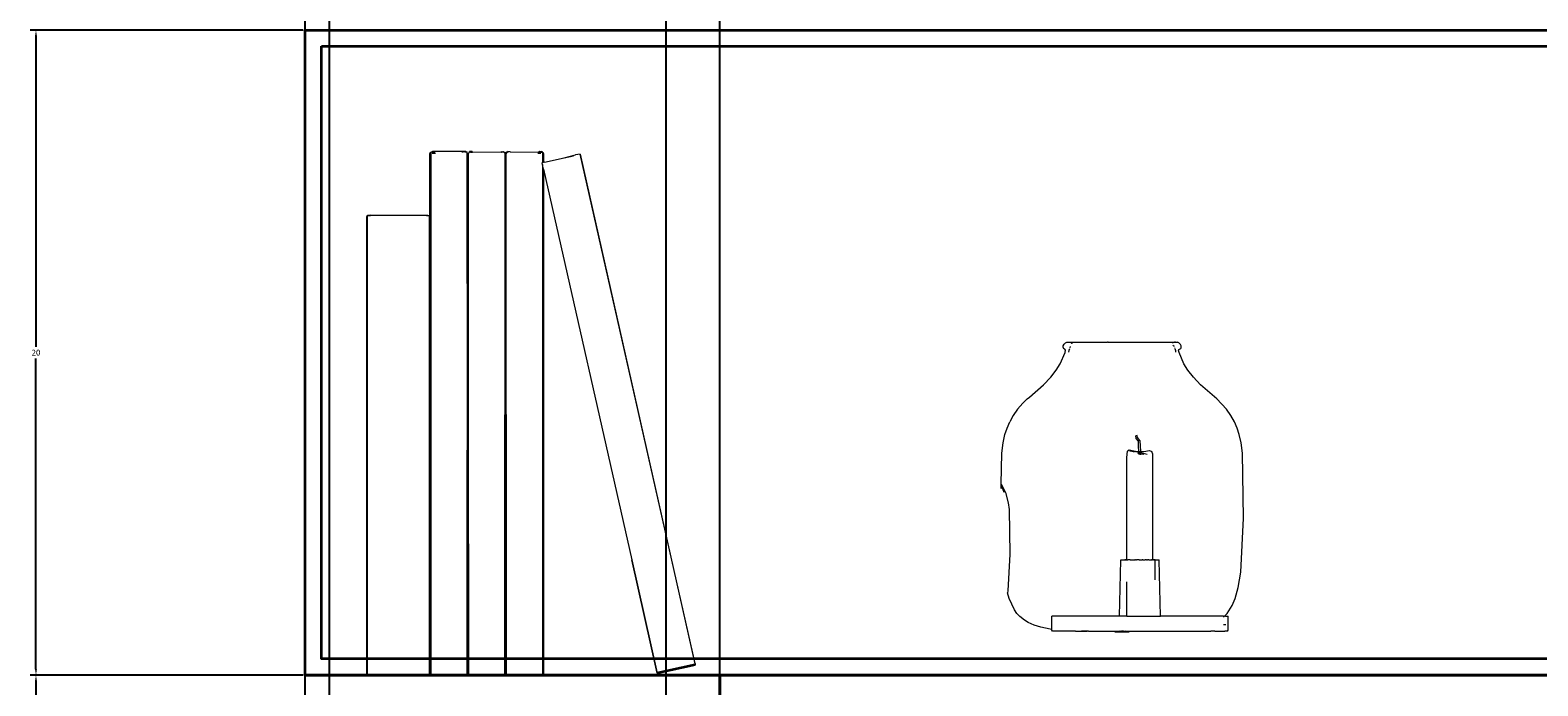
# Model space of a CAD drawing. Units: millimetres. Extents: x 446512 to 447461, y 70395 to 70610.
# Tile 18 of 39: x 446678 to 446725, y 70513 to 70533. Entities that reach past the tile are written whole.
import ezdxf

# ---------------------------------------------------------------- set-up
doc = ezdxf.new("R2010")
doc.units = ezdxf.units.MM
for name, color, linetype, lineweight in [('A-ANNO-DIMS', 2, 'Continuous', 18), ('A-CONS', 9, 'Continuous', 13), ('A-FURN', 7, 'Continuous', 35), ('A-FURN-DECO', 8, 'Continuous', 13)]:
    doc.layers.add(name, color=color, linetype=linetype, lineweight=lineweight)
doc.styles.get("Standard").update_dxf_attribs({"font": 'arial.ttf'})
doc.dimstyles.get("Standard").update_dxf_attribs({"dimtxt": 0.18, "dimasz": 0.18, "dimexe": 0.18, "dimexo": 0.0625, "dimgap": 0.09, "dimtad": 0, "dimtih": 1, "dimtoh": 1, "dimdec": 4, "dimzin": 0, "dimdsep": 46, "dimtxsty": 'Standard', "dimcen": 0.09, "dimadec": 0, "dimazin": 0, "dimtfac": 1, "dimtdec": 4, "dimtofl": 0, "dimtmove": 0, "dimatfit": 3, "dimfxl": 1, "dimtolj": 1, "dimtzin": 0, "dimarcsym": 0})

# ---------------------------------------------------------------- blocks, each defined once
blk = doc.blocks.new('DECO-VASE-A')
for p, q in [((1.923, 8.866), (1.951, 8.922)), ((1.951, 8.922), (1.992, 8.962)), ((1.992, 8.962), (2.04, 8.983)), ((2.04, 8.983), (2.147, 8.974)), ((2.04, 8.983), (3.3, 8.983)), ((2.147, 8.974), (2.186, 8.942)), ((2.186, 8.942), (2.19, 8.923)), ((3.314, 8.982), (3.3, 8.983)), ((3.314, 8.982), (5.399, 8.983)), ((5.308, 8.977), (5.375, 8.979)), ((5.332, 8.964), (5.314, 8.943)), ((5.325, 8.885), (5.351, 8.865)), ((5.375, 8.979), (5.332, 8.964)), ((5.399, 8.983), (5.375, 8.979)), ((5.403, 8.983), (5.399, 8.983)), ((5.403, 8.983), (5.462, 8.982)), ((5.511, 8.96), (5.462, 8.982)), ((5.56, 8.904), (5.511, 8.96)), ((5.576, 8.866), (5.56, 8.904)), ((1.832, 8.302), (1.985, 8.655)), ((1.917, 8.815), (1.923, 8.866)), ((1.917, 8.815), (1.931, 8.786)), ((1.974, 8.762), (1.931, 8.786)), ((1.996, 8.731), (1.974, 8.762)), ((1.985, 8.655), (1.996, 8.731)), ((2.1, 8.723), (2.091, 8.673)), ((2.115, 8.769), (2.1, 8.723)), ((2.141, 8.848), (2.125, 8.798)), ((5.351, 8.865), (5.358, 8.847)), ((5.373, 8.802), (5.377, 8.793)), ((5.382, 8.778), (5.4, 8.725)), ((5.4, 8.725), (5.409, 8.672)), ((5.503, 8.731), (5.511, 8.747)), ((5.515, 8.655), (5.503, 8.731)), ((5.511, 8.747), (5.566, 8.783)), ((5.668, 8.302), (5.515, 8.655)), ((5.566, 8.783), (5.581, 8.808)), ((5.581, 8.808), (5.576, 8.866)), ((1.541, 7.898), (1.71, 8.114)), ((1.71, 8.114), (1.832, 8.302)), ((5.789, 8.114), (5.668, 8.302)), ((5.959, 7.898), (5.789, 8.114)), ((0.874, 7.277), (1.315, 7.659)), ((1.315, 7.659), (1.541, 7.898)), ((6.185, 7.659), (5.959, 7.898)), ((6.689, 7.222), (6.185, 7.659)), ((0.508, 6.898), (0.67, 7.084)), ((0.67, 7.084), (0.81, 7.222)), ((0.81, 7.222), (0.874, 7.277)), ((6.991, 6.898), (6.689, 7.222)), ((0.375, 6.707), (0.267, 6.512)), ((0.508, 6.898), (0.375, 6.707)), ((7.124, 6.707), (6.991, 6.898)), ((7.232, 6.512), (7.124, 6.707)), ((0.06, 5.856), (0.117, 6.113)), ((0.117, 6.113), (0.182, 6.314)), ((0.182, 6.314), (0.267, 6.512)), ((4.217, 6.081), (4.173, 6.078)), ((4.184, 5.991), (4.173, 6.078)), ((4.227, 6.021), (4.217, 6.081)), ((7.317, 6.314), (7.232, 6.512)), ((7.382, 6.113), (7.317, 6.314)), ((7.44, 5.856), (7.382, 6.113)), ((0.02, 5.541), (0.06, 5.856)), ((3.97, 5.625), (3.916, 5.6)), ((4.168, 5.588), (3.97, 5.625)), ((4.129, 5.567), (3.989, 5.611)), ((3.989, 5.611), (4.168, 5.588)), ((4.258, 5.909), (4.184, 5.991)), ((4.297, 5.928), (4.227, 6.021)), ((4.261, 5.759), (4.258, 5.909)), ((4.266, 5.588), (4.261, 5.759)), ((4.297, 5.928), (4.32, 5.588)), ((4.422, 5.588), (4.602, 5.615)), ((4.602, 5.615), (4.675, 5.587)), ((7.479, 5.541), (7.44, 5.856)), ((0.002, 4.579), (0.02, 5.541)), ((3.893, 5.401), (3.916, 5.6)), ((3.893, 2.225), (3.893, 5.401)), ((4.168, 5.588), (4.266, 5.588)), ((4.267, 5.562), (4.168, 5.588)), ((4.268, 5.524), (4.24, 5.533)), ((4.267, 5.562), (4.266, 5.588)), ((4.266, 5.588), (4.32, 5.588)), ((4.322, 5.548), (4.267, 5.562)), ((4.267, 5.554), (4.267, 5.559)), ((4.268, 5.524), (4.267, 5.541)), ((4.295, 5.515), (4.268, 5.524)), ((4.268, 5.504), (4.268, 5.524)), ((4.303, 5.503), (4.268, 5.504)), ((4.295, 5.515), (4.325, 5.513)), ((4.303, 5.503), (4.325, 5.502)), ((4.32, 5.588), (4.322, 5.548)), ((4.32, 5.588), (4.422, 5.588)), ((4.525, 5.496), (4.322, 5.548)), ((4.323, 5.541), (4.324, 5.523)), ((4.325, 5.513), (4.325, 5.502)), ((4.325, 5.513), (4.428, 5.504)), ((4.691, 5.523), (4.675, 5.587)), ((4.691, 5.523), (4.695, 2.225)), ((7.516, 3.52), (7.479, 5.541)), ((0, 4.513), (0.002, 4.579)), ((0.002, 4.51), (0, 4.513)), ((0, 4.439), (0.002, 4.51)), ((0.002, 4.579), (0.134, 4.312)), ((0.052, 4.428), (0.002, 4.51)), ((0.095, 4.312), (0.052, 4.428)), ((0.134, 4.312), (0.217, 3.999)), ((0.217, 3.999), (0.244, 3.785)), ((0.244, 3.785), (0.269, 2.409)), ((7.431, 1.848), (7.516, 3.52)), ((0.269, 2.409), (0.211, 1.27)), ((3.665, 0.487), (3.705, 2.219)), ((3.705, 2.219), (3.712, 2.225)), ((3.712, 2.225), (3.763, 2.225)), ((3.763, 2.225), (3.766, 2.225)), ((3.766, 2.225), (3.789, 2.225)), ((3.789, 2.225), (3.795, 2.225)), ((3.795, 2.225), (3.797, 2.225)), ((3.797, 2.225), (3.813, 2.225)), ((3.813, 2.225), (3.821, 2.225)), ((3.821, 2.225), (3.825, 2.225)), ((3.825, 2.225), (3.828, 2.225)), ((3.828, 2.225), (3.832, 2.225)), ((3.832, 2.225), (3.838, 2.225)), ((3.842, 2.225), (3.838, 2.225)), ((3.838, 2.225), (3.838, 2.219)), ((3.842, 2.225), (3.844, 2.225)), ((3.844, 2.225), (3.852, 2.225)), ((3.864, 2.225), (3.852, 2.225)), ((3.867, 2.225), (3.864, 2.225)), ((3.867, 2.225), (3.878, 2.225)), ((3.878, 2.225), (3.881, 2.225)), ((3.881, 2.225), (3.883, 2.225)), ((3.883, 2.225), (3.893, 2.225)), ((3.893, 2.219), (3.893, 2.225)), ((3.908, 2.225), (3.893, 2.225)), ((3.908, 2.225), (3.927, 2.225)), ((3.992, 2.225), (3.927, 2.225)), ((4.002, 2.225), (3.992, 2.225)), ((4.002, 2.225), (4.053, 2.225)), ((4.053, 2.225), (4.065, 2.225)), ((4.065, 2.225), (4.148, 2.225)), ((4.163, 2.225), (4.148, 2.225)), ((4.163, 2.225), (4.192, 2.225)), ((4.278, 2.225), (4.192, 2.225)), ((4.278, 2.225), (4.283, 2.225)), ((4.283, 2.225), (4.374, 2.225)), ((4.394, 2.225), (4.374, 2.225)), ((4.394, 2.225), (4.451, 2.225)), ((4.451, 2.225), (4.462, 2.225)), ((4.496, 2.225), (4.462, 2.225)), ((4.5, 2.225), (4.496, 2.225)), ((4.505, 2.225), (4.5, 2.225)), ((4.505, 2.225), (4.508, 2.225)), ((4.508, 2.225), (4.511, 2.225)), ((4.511, 2.225), (4.541, 2.225)), ((4.553, 2.225), (4.541, 2.225)), ((4.578, 2.225), (4.553, 2.225)), ((4.578, 2.225), (4.583, 2.225)), ((4.583, 2.225), (4.65, 2.225)), ((4.659, 2.225), (4.65, 2.225)), ((4.659, 2.225), (4.683, 2.225)), ((4.69, 2.225), (4.683, 2.225)), ((4.695, 2.225), (4.69, 2.225)), ((4.695, 2.225), (4.695, 2.219)), ((4.697, 2.225), (4.695, 2.225)), ((4.702, 2.225), (4.697, 2.225)), ((4.704, 2.225), (4.702, 2.225)), ((4.704, 2.225), (4.718, 2.225)), ((4.722, 2.225), (4.718, 2.225)), ((4.74, 2.225), (4.722, 2.225)), ((4.744, 2.225), (4.74, 2.225)), ((4.744, 2.225), (4.756, 2.225)), ((4.769, 2.225), (4.756, 2.225)), ((4.769, 2.225), (4.76, 1.611)), ((4.773, 2.225), (4.769, 2.225)), ((4.777, 2.225), (4.773, 2.225)), ((4.777, 2.225), (4.802, 2.225)), ((4.802, 2.225), (4.807, 2.225)), ((4.807, 2.225), (4.813, 2.225)), ((4.813, 2.225), (4.834, 2.225)), ((4.834, 2.225), (4.837, 2.225)), ((4.837, 2.225), (4.84, 2.225)), ((4.84, 2.225), (4.849, 2.225)), ((4.849, 2.225), (4.895, 2.225)), ((4.902, 2.219), (4.895, 2.225)), ((4.942, 0.487), (4.902, 2.219)), ((3.893, 0.487), (3.893, 1.548)), ((7.347, 1.371), (7.431, 1.848)), ((0.211, 1.27), (0.2, 1.204)), ((0.248, 1.032), (0.2, 1.204)), ((0.41, 0.681), (0.248, 1.032)), ((7.16, 0.81), (7.251, 1.032)), ((7.251, 1.032), (7.347, 1.371)), ((0.488, 0.567), (0.41, 0.681)), ((0.576, 0.472), (0.488, 0.567)), ((0.727, 0.355), (0.576, 0.472)), ((1.567, 0.24), (1.568, 0.487)), ((3.665, 0.487), (1.568, 0.487)), ((3.893, 0.487), (3.665, 0.487)), ((3.893, 0.487), (4.942, 0.487)), ((6.889, 0.487), (4.942, 0.487)), ((6.889, 0.452), (6.926, 0.487)), ((6.889, 0.487), (6.926, 0.487)), ((6.926, 0.487), (7.011, 0.567)), ((6.938, 0.487), (6.926, 0.487)), ((6.953, 0.487), (6.938, 0.487)), ((6.953, 0.487), (7.039, 0.487)), ((7.011, 0.567), (7.16, 0.81)), ((7.039, 0.045), (7.039, 0.487)), ((0.839, 0.288), (0.727, 0.355)), ((1.025, 0.205), (0.839, 0.288)), ((1.227, 0.14), (1.025, 0.205)), ((1.518, 0.077), (1.227, 0.14)), ((1.567, 0.071), (1.518, 0.077)), ((1.567, 0.071), (1.567, 0.24)), ((1.567, 0.045), (1.567, 0.071)), ((1.588, 0.02), (1.567, 0.045)), ((2.274, 0.02), (1.588, 0.02)), ((2.295, 0.021), (2.274, 0.02)), ((2.306, 0.02), (2.295, 0.021)), ((2.306, 0.02), (2.665, 0.02)), ((2.665, 0.02), (2.495, 0.021)), ((2.684, 0.022), (2.665, 0.02)), ((2.704, 0.02), (2.684, 0.022)), ((2.704, 0.02), (3.676, 0.02)), ((3.521, 0), (3.685, 0.017)), ((3.521, 0), (3.97, 0)), ((3.685, 0.017), (3.676, 0.02)), ((3.685, 0.017), (3.729, 0.02)), ((3.775, 0.017), (3.729, 0.02)), ((3.793, 0.02), (3.775, 0.017)), ((3.793, 0.02), (3.84, 0.017)), ((3.84, 0.017), (3.859, 0.02)), ((3.97, 0), (3.84, 0.017)), ((3.859, 0.02), (6.333, 0.02)), ((6.333, 0.02), (6.501, 0.021)), ((6.622, 0.02), (6.501, 0.021)), ((6.622, 0.02), (6.643, 0.02)), ((6.643, 0.02), (6.645, 0.02)), ((6.643, 0.02), (6.647, 0.02)), ((6.647, 0.02), (6.749, 0.02)), ((6.749, 0.02), (6.768, 0.02)), ((6.768, 0.02), (6.77, 0.02)), ((6.77, 0.02), (6.854, 0.02)), ((6.854, 0.02), (6.911, 0.02)), ((6.911, 0.02), (6.933, 0.02)), ((6.945, 0.02), (6.933, 0.02)), ((7.019, 0.02), (6.945, 0.02)), ((7.019, 0.02), (7.039, 0.045))]:
    blk.add_line(p, q)
blk = doc.blocks.new('*D22')
at = {"layer": 'A-ANNO-DIMS', "color": 0, "lineweight": -2, "transparency": 16777216}
for p, q in [((446686.51, 70513.382), (446678.043, 70513.382)), ((446678.223, 70513.202), (446678.223, 70503.563)), ((446678.223, 70493.562), (446678.223, 70503.2)), ((446686.51, 70493.382), (446678.043, 70493.382))]:
    blk.add_line(p, q, dxfattribs=at)
at = {"layer": 'A-ANNO-DIMS', "color": 0, "transparency": 16777216}
for points in [[(446678.193, 70513.202), (446678.253, 70513.202), (446678.223, 70513.382)], [(446678.193, 70493.562), (446678.253, 70493.562), (446678.223, 70493.382)]]:
    blk.add_solid(points, dxfattribs=at)
at = {"layer": 'Defpoints', "color": 0, "transparency": 16777216}
for p in [(446678.223, 70513.382), (446686.573, 70513.382), (446686.573, 70493.382)]:
    blk.add_point(p, dxfattribs=at)
at = {"layer": 'A-ANNO-DIMS', "color": 0, "transparency": 16777216, "insert": (446678.223, 70503.382), "char_height": 0.18, "attachment_point": 5}
blk.add_mtext('\\A1;20', dxfattribs=at)
blk = doc.blocks.new('*D23')
at = {"layer": 'A-ANNO-DIMS', "color": 0, "lineweight": -2, "transparency": 16777216}
for p, q in [((446686.51, 70533.382), (446678.043, 70533.382)), ((446678.223, 70533.202), (446678.223, 70523.563)), ((446678.223, 70513.562), (446678.223, 70523.2)), ((446686.51, 70513.382), (446678.043, 70513.382))]:
    blk.add_line(p, q, dxfattribs=at)
at = {"layer": 'A-ANNO-DIMS', "color": 0, "transparency": 16777216}
for points in [[(446678.193, 70533.202), (446678.253, 70533.202), (446678.223, 70533.382)], [(446678.193, 70513.562), (446678.253, 70513.562), (446678.223, 70513.382)]]:
    blk.add_solid(points, dxfattribs=at)
at = {"layer": 'Defpoints', "color": 0, "transparency": 16777216}
for p in [(446678.223, 70533.382), (446686.573, 70533.382), (446686.573, 70513.382)]:
    blk.add_point(p, dxfattribs=at)
at = {"layer": 'A-ANNO-DIMS', "color": 0, "transparency": 16777216, "insert": (446678.223, 70523.382), "char_height": 0.18, "attachment_point": 5}
blk.add_mtext('\\A1;20', dxfattribs=at)
blk = doc.blocks.new('*D37')
at = {"layer": 'A-ANNO-DIMS', "color": 0, "lineweight": -2, "transparency": 16777216}
for p, q in [((446686.572846, 70433.44405), (446686.572846, 70578.17492)), ((446687.323552, 70428.838404), (446687.323552, 70578.17492)), ((446686.392846, 70577.99492), (446686.212846, 70577.99492)), ((446687.503552, 70577.99492), (446687.683552, 70577.99492))]:
    blk.add_line(p, q, dxfattribs=at)
at = {"layer": 'A-ANNO-DIMS', "color": 0, "transparency": 16777216}
for points in [[(446686.392846, 70578.02492), (446686.392846, 70577.96492), (446686.572846, 70577.99492)], [(446687.503552, 70578.02492), (446687.503552, 70577.96492), (446687.323552, 70577.99492)]]:
    blk.add_solid(points, dxfattribs=at)
at = {"layer": 'Defpoints', "color": 0, "transparency": 16777216}
for p in [(446687.323552, 70577.99492), (446686.572846, 70433.38155), (446687.323552, 70428.775904)]:
    blk.add_point(p, dxfattribs=at)
at = {"layer": 'A-ANNO-DIMS', "color": 0, "transparency": 16777216, "insert": (446686.948199, 70577.99492), "char_height": 0.18, "attachment_point": 5}
blk.add_mtext('\\A1;0.75', dxfattribs=at)
blk = doc.blocks.new('*D38')
at = {"layer": 'A-ANNO-DIMS', "color": 0, "lineweight": -2, "transparency": 16777216}
for p, q in [((446687.323552, 70428.838404), (446687.323552, 70578.17492)), ((446697.765686, 70428.838404), (446697.765686, 70578.17492)), ((446687.503552, 70577.99492), (446692.090383, 70577.99492)), ((446697.585686, 70577.99492), (446692.998855, 70577.99492))]:
    blk.add_line(p, q, dxfattribs=at)
at = {"layer": 'A-ANNO-DIMS', "color": 0, "transparency": 16777216}
for points in [[(446687.503552, 70578.02492), (446687.503552, 70577.96492), (446687.323552, 70577.99492)], [(446697.585686, 70578.02492), (446697.585686, 70577.96492), (446697.765686, 70577.99492)]]:
    blk.add_solid(points, dxfattribs=at)
at = {"layer": 'Defpoints', "color": 0, "transparency": 16777216}
for p in [(446697.765686, 70577.99492), (446687.323552, 70428.775904), (446697.765686, 70428.775904)]:
    blk.add_point(p, dxfattribs=at)
at = {"layer": 'A-ANNO-DIMS', "color": 0, "transparency": 16777216, "insert": (446692.544619, 70577.99492), "char_height": 0.18, "attachment_point": 5}
blk.add_mtext('\\A1;10.442', dxfattribs=at)
blk = doc.blocks.new('*D39')
at = {"layer": 'A-ANNO-DIMS', "color": 0, "lineweight": -2, "transparency": 16777216}
for p, q in [((446697.766, 70428.838), (446697.766, 70578.175)), ((446699.429, 70433.444), (446699.429, 70578.175)), ((446697.946, 70577.995), (446698.212, 70577.995)), ((446699.249, 70577.995), (446698.982, 70577.995))]:
    blk.add_line(p, q, dxfattribs=at)
at = {"layer": 'A-ANNO-DIMS', "color": 0, "transparency": 16777216}
for points in [[(446697.946, 70578.025), (446697.946, 70577.965), (446697.766, 70577.995)], [(446699.249, 70578.025), (446699.249, 70577.965), (446699.429, 70577.995)]]:
    blk.add_solid(points, dxfattribs=at)
at = {"layer": 'Defpoints', "color": 0, "transparency": 16777216}
for p in [(446699.429, 70577.995), (446699.429, 70433.382), (446697.766, 70428.776)]:
    blk.add_point(p, dxfattribs=at)
at = {"layer": 'A-ANNO-DIMS', "color": 0, "transparency": 16777216, "insert": (446698.597, 70577.995), "char_height": 0.18, "attachment_point": 5}
blk.add_mtext('\\A1;1.663', dxfattribs=at)

msp = doc.modelspace()

# ---------------------------------------------------------------- linework, layer by layer
at = {"layer": 'A-CONS'}
msp.add_point((446686.5728, 70513.3815), dxfattribs=at)
at = {"layer": 'A-FURN'}
for p, q in [((446686.5728, 70533.3815), (446746.5728, 70533.3815)), ((446686.5728, 70513.3815), (446686.5728, 70533.3815)), ((446686.5728, 70533.3815), (446729.0084, 70533.3815)), ((446686.5728, 70513.3815), (446686.5728, 70533.3815)), ((446698.6596, 70513.705), (446697.4869, 70513.4397)), ((446686.5728, 70513.3815), (446746.5728, 70513.3815)), ((446729.0084, 70513.3815), (446686.5728, 70513.3815)), ((446688.4996, 70513.3815), (446693.9312, 70513.3815)), ((446699.4288, 70513.3815), (446699.4288, 70493.3815))]:
    msp.add_line(p, q, dxfattribs=at)
for points in [[(446687.0728, 70532.8815), (446728.5084, 70532.8815), (446728.5084, 70513.8815), (446687.0728, 70513.8815)], [(446699.4288, 70513.3815), (446746.5728, 70513.3815), (446746.5728, 70493.3815), (446699.4288, 70493.3815)]]:
    msp.add_lwpolyline(points, close=True, dxfattribs=at)
at = {"layer": 'A-FURN-DECO'}
for p, q in [((446690.4351, 70529.5416), (446690.4536, 70529.596)), ((446690.4536, 70529.5838), (446690.4351, 70529.5416)), ((446690.4351, 70513.4359), (446690.4351, 70529.5416)), ((446690.4536, 70529.596), (446690.4589, 70529.596)), ((446690.4536, 70529.596), (446690.4536, 70529.5838)), ((446690.4589, 70529.596), (446690.4536, 70529.5838)), ((446690.4536, 70529.5838), (446690.4536, 70529.5517)), ((446690.4589, 70529.596), (446690.4655, 70529.596)), ((446690.4655, 70529.596), (446690.4645, 70513.3815)), ((446690.4655, 70529.596), (446690.4738, 70529.5992)), ((446690.4738, 70529.5992), (446690.5121, 70529.6141)), ((446690.4931, 70529.6009), (446690.4738, 70529.5992)), ((446690.4738, 70529.5992), (446690.4862, 70529.596)), ((446690.4957, 70529.6027), (446690.4931, 70529.6009)), ((446691.5463, 70529.6141), (446690.5121, 70529.6141)), ((446690.5309, 70529.5424), (446690.5293, 70529.596)), ((446690.5346, 70529.5426), (446690.5346, 70529.596)), ((446690.5644, 70529.596), (446690.5708, 70529.5445)), ((446690.5644, 70529.5442), (446690.5644, 70529.596)), ((446690.5644, 70529.596), (446690.5669, 70529.5443)), ((446690.5829, 70529.596), (446690.5868, 70529.5454)), ((446691.4454, 70529.5918), (446691.4453, 70529.596)), ((446691.4532, 70529.596), (446691.4453, 70529.596)), ((446691.476, 70529.5935), (446691.4762, 70529.5968)), ((446691.481, 70529.596), (446691.4808, 70529.5937)), ((446691.5107, 70529.596), (446691.481, 70529.596)), ((446691.5347, 70529.605), (446691.5864, 70529.596)), ((446691.5463, 70529.6141), (446691.5881, 70529.596)), ((446691.5881, 70529.596), (446691.5864, 70529.596)), ((446691.5911, 70529.5416), (446691.5881, 70529.596)), ((446691.5918, 70529.596), (446691.5881, 70529.596)), ((446691.5911, 70529.5416), (446691.5898, 70527.3506)), ((446691.5911, 70529.5416), (446691.5918, 70529.596)), ((446691.6103, 70513.4359), (446691.5911, 70529.5416)), ((446691.6103, 70529.5416), (446691.6535, 70529.5885)), ((446691.6293, 70516.6542), (446691.6103, 70529.5416)), ((446691.6103, 70529.5416), (446691.6294, 70513.4359)), ((446691.6288, 70529.5416), (446691.6535, 70529.5885)), ((446691.6293, 70516.6542), (446691.6288, 70529.5416)), ((446691.6535, 70529.5885), (446691.6604, 70529.596)), ((446691.6604, 70529.596), (446691.667, 70529.6141)), ((446691.6604, 70529.596), (446691.7069, 70529.6062)), ((446691.7466, 70529.6141), (446691.667, 70529.6141)), ((446691.6974, 70529.596), (446691.7397, 70529.5968)), ((446691.7402, 70529.5996), (446691.7397, 70529.5968)), ((446691.7397, 70529.5968), (446691.7574, 70529.5971)), ((446691.7574, 70529.5971), (446691.7466, 70529.6141)), ((446691.7574, 70529.5971), (446692.6506, 70529.6131)), ((446692.6478, 70529.596), (446692.6562, 70529.596)), ((446692.6525, 70529.6141), (446692.6506, 70529.6131)), ((446692.6543, 70529.6132), (446692.6525, 70529.6141)), ((446692.6543, 70529.6132), (446692.7084, 70529.6141)), ((446692.6562, 70529.596), (446692.6557, 70529.5984)), ((446692.6859, 70529.596), (446692.6562, 70529.596)), ((446692.6859, 70529.596), (446692.6724, 70529.6033)), ((446692.6912, 70529.596), (446692.6859, 70529.596)), ((446692.6885, 70529.6082), (446692.7008, 70529.6061)), ((446692.7008, 70529.6061), (446692.6912, 70529.596)), ((446692.7084, 70529.6141), (446692.7008, 70529.6061)), ((446692.7008, 70529.6061), (446692.7259, 70529.6019)), ((446692.7084, 70529.6141), (446692.7259, 70529.6019)), ((446692.7259, 70529.6019), (446692.7344, 70529.596)), ((446692.7259, 70529.6019), (446692.7616, 70529.596)), ((446692.76, 70529.5523), (446692.7344, 70529.596)), ((446692.756, 70513.3815), (446692.7663, 70529.5416)), ((446692.76, 70529.5523), (446692.7616, 70529.5516)), ((446692.7663, 70529.5416), (446692.76, 70529.5523)), ((446692.7854, 70529.5416), (446692.7616, 70529.596)), ((446692.7616, 70513.3815), (446692.7854, 70529.5416)), ((446692.767, 70513.3815), (446692.7854, 70529.5416)), ((446692.7854, 70529.5416), (446692.8039, 70529.596)), ((446692.8092, 70529.596), (446692.7854, 70529.5416)), ((446692.7854, 70513.4359), (446692.7854, 70529.5416)), ((446692.7854, 70529.5416), (446692.8039, 70513.3938)), ((446692.8039, 70529.596), (446692.8092, 70529.596)), ((446692.8039, 70529.5416), (446692.8364, 70529.596)), ((446692.8076, 70513.3853), (446692.8039, 70529.5416)), ((446692.8092, 70529.596), (446692.8394, 70529.601)), ((446692.8364, 70529.596), (446692.8092, 70529.596)), ((446692.8364, 70529.596), (446692.8394, 70529.601)), ((446692.8725, 70529.596), (446692.8364, 70529.596)), ((446692.8394, 70529.601), (446692.8472, 70529.6141)), ((446692.8394, 70529.601), (446692.8606, 70529.6045)), ((446692.9162, 70529.6129), (446692.8472, 70529.6141)), ((446692.9148, 70529.5937), (446692.9147, 70529.596)), ((446692.9184, 70529.6141), (446692.9162, 70529.6129)), ((446692.9162, 70529.6129), (446692.9203, 70529.6129)), ((446692.9184, 70529.6141), (446692.9203, 70529.6129)), ((446692.9191, 70529.5935), (446692.919, 70529.596)), ((446692.9203, 70529.6129), (446693.7956, 70529.596)), ((446692.9462, 70529.592), (446692.9463, 70529.596)), ((446693.7956, 70529.596), (446693.7941, 70529.5462)), ((446693.7956, 70529.596), (446693.7989, 70529.5979)), ((446693.7989, 70529.5979), (446693.8276, 70529.6141)), ((446693.7989, 70529.5979), (446693.827, 70529.5974)), ((446693.827, 70529.5974), (446693.825, 70529.5445)), ((446693.8276, 70529.6141), (446693.827, 70529.5974)), ((446693.827, 70529.5974), (446693.831, 70529.5973)), ((446693.8276, 70529.6141), (446693.831, 70529.5973)), ((446693.8595, 70529.5968), (446693.8276, 70529.6141)), ((446693.8276, 70529.6141), (446693.8988, 70529.6141)), ((446693.8276, 70529.6141), (446693.8749, 70529.6037)), ((446693.8799, 70529.6058), (446693.8276, 70529.6141)), ((446693.831, 70529.5973), (446693.8288, 70529.5443)), ((446693.831, 70529.5973), (446693.8313, 70529.5442)), ((446693.831, 70529.5973), (446693.8595, 70529.5968)), ((446693.8595, 70529.5968), (446693.8631, 70529.596)), ((446693.8595, 70529.5968), (446693.861, 70529.596)), ((446693.861, 70529.5426), (446693.861, 70529.596)), ((446693.861, 70529.5426), (446693.8631, 70529.596)), ((446693.861, 70529.596), (446693.8631, 70529.596)), ((446693.8631, 70529.596), (446693.8646, 70529.5968)), ((446693.8631, 70529.596), (446693.9095, 70529.596)), ((446693.8646, 70529.5968), (446693.8749, 70529.6037)), ((446693.8749, 70529.6037), (446693.8772, 70529.6032)), ((446693.8772, 70529.6032), (446693.8799, 70529.6058)), ((446693.8772, 70529.6032), (446693.9095, 70529.596)), ((446693.8818, 70529.6055), (446693.8799, 70529.6058)), ((446693.8818, 70529.6055), (446693.8988, 70529.6141)), ((446693.9256, 70529.5986), (446693.8818, 70529.6055)), ((446693.9256, 70529.5986), (446693.8988, 70529.6141)), ((446693.9095, 70529.596), (446693.9256, 70529.5986)), ((446693.9301, 70529.596), (446693.9256, 70529.5986)), ((446693.9301, 70529.596), (446693.9302, 70529.2759)), ((446693.9421, 70529.596), (446693.9301, 70529.596)), ((446693.9421, 70529.596), (446693.9606, 70529.5416)), ((446693.9421, 70529.5517), (446693.9421, 70529.596)), ((446693.9606, 70529.5416), (446693.9606, 70529.29)), ((446694.6035, 70529.4244), (446694.9523, 70529.5154)), ((446694.6035, 70529.4244), (446694.886, 70529.4881)), ((446695.0903, 70529.5341), (446694.9523, 70529.5154)), ((446695.0922, 70529.5345), (446695.0903, 70529.5341)), ((446695.0903, 70529.5341), (446698.6538, 70513.7305)), ((446698.6645, 70513.7432), (446695.0922, 70529.5345)), ((446693.9188, 70529.2701), (446693.9302, 70529.2759)), ((446693.9188, 70529.2701), (446693.9304, 70529.2727)), ((446693.9302, 70529.2198), (446693.9188, 70529.2701)), ((446693.9302, 70529.2759), (446693.9606, 70529.29)), ((446693.9302, 70529.2759), (446693.9304, 70529.2727)), ((446693.9302, 70529.2198), (446693.9302, 70529.2108)), ((446693.9302, 70529.2108), (446693.9312, 70513.3815)), ((446693.9621, 70529.0693), (446693.9302, 70529.2108)), ((446693.9928, 70529.2868), (446693.9304, 70529.2727)), ((446693.9685, 70529.2937), (446693.9606, 70529.29)), ((446693.9606, 70529.29), (446693.9606, 70529.2842)), ((446693.9621, 70529.0693), (446693.9606, 70513.4359)), ((446693.9621, 70529.0693), (446696.6945, 70516.9532)), ((446693.9685, 70529.2937), (446693.9928, 70529.2868)), ((446693.9928, 70529.2868), (446694.6035, 70529.4244)), ((446688.4765, 70527.5829), (446688.491, 70527.629)), ((446688.491, 70527.6186), (446688.4765, 70527.5829)), ((446688.491, 70527.629), (446688.4952, 70527.629)), ((446688.491, 70527.629), (446688.491, 70527.6186)), ((446688.4952, 70527.629), (446688.491, 70527.6186)), ((446688.491, 70527.6186), (446688.491, 70527.5915)), ((446688.4952, 70527.629), (446688.4996, 70527.629)), ((446688.4996, 70527.629), (446688.5057, 70527.6315)), ((446688.4996, 70513.3815), (446688.4996, 70527.629)), ((446688.5057, 70527.6315), (446688.5369, 70527.6443)), ((446688.5057, 70527.6315), (446688.5429, 70527.6375)), ((446688.5504, 70527.629), (446688.5057, 70527.6315)), ((446688.5369, 70527.6443), (446688.5808, 70527.6443)), ((446688.5429, 70527.6375), (446688.5369, 70527.6443)), ((446688.5429, 70527.6375), (446688.5808, 70527.6443)), ((446688.5504, 70527.629), (446688.5429, 70527.6375)), ((446688.5504, 70527.629), (446688.5712, 70527.629)), ((446688.5712, 70527.629), (446688.5809, 70527.6412)), ((446688.5779, 70527.629), (446688.5712, 70527.629)), ((446688.5779, 70527.629), (446688.5809, 70527.6412)), ((446688.5779, 70527.629), (446688.5813, 70527.629)), ((446688.5834, 70527.6443), (446688.5808, 70527.6443)), ((446688.5809, 70527.6412), (446688.5808, 70527.6443)), ((446688.5813, 70527.629), (446688.5809, 70527.6412)), ((446688.5809, 70527.6412), (446688.6059, 70527.629)), ((446688.6059, 70527.629), (446688.5813, 70527.629)), ((446688.6059, 70527.629), (446688.5834, 70527.6443)), ((446688.5834, 70527.6443), (446690.3747, 70527.6443)), ((446690.3157, 70527.629), (446688.6059, 70527.629)), ((446690.3192, 70527.629), (446690.3157, 70527.629)), ((446690.3337, 70527.629), (446690.3192, 70527.629)), ((446690.3337, 70527.629), (446690.3747, 70527.6443)), ((446690.3337, 70527.629), (446690.3571, 70527.629)), ((446690.3571, 70527.629), (446690.3612, 70527.629)), ((446690.3594, 70527.629), (446690.3571, 70527.629)), ((446690.3612, 70527.629), (446690.3594, 70527.629)), ((446690.3747, 70527.6443), (446690.3612, 70527.629)), ((446690.3612, 70527.629), (446690.3666, 70527.629)), ((446690.3666, 70527.629), (446690.4164, 70527.629)), ((446690.3747, 70527.6443), (446690.4164, 70527.629)), ((446690.4206, 70527.629), (446690.4164, 70527.629)), ((446690.4201, 70527.5829), (446690.4164, 70527.629)), ((446690.4201, 70527.5829), (446690.4206, 70527.629)), ((446688.4765, 70513.4248), (446688.4765, 70527.5829)), ((446690.4201, 70527.5829), (446690.4174, 70526.8795)), ((446690.4351, 70513.4359), (446690.4201, 70527.5829)), ((446691.5898, 70527.3506), (446691.5809, 70513.3815)), ((446691.5898, 70527.3506), (446691.6103, 70513.4359)), ((446690.4174, 70526.8795), (446690.4208, 70524.2798)), ((446690.4208, 70524.2798), (446690.4121, 70513.3815)), ((446690.4208, 70524.2798), (446690.4351, 70513.4359)), ((446690.4215, 70513.3913), (446690.4208, 70524.2798)), ((446696.6945, 70516.9532), (446697.4842, 70513.4401)), ((446697.4867, 70513.4407), (446696.6945, 70516.9532)), ((446715.0887, 70514.9372), (446715.0374, 70514.9369)), ((446715.1132, 70514.9372), (446715.0887, 70514.9372)), ((446698.5372, 70513.6774), (446698.1698, 70513.5822)), ((446698.5372, 70513.6774), (446698.6577, 70513.7045)), ((446698.6596, 70513.705), (446698.6538, 70513.7305)), ((446698.6538, 70513.7305), (446698.6577, 70513.7045)), ((446698.6596, 70513.705), (446698.6577, 70513.7045)), ((446698.6645, 70513.7432), (446698.6596, 70513.705)), ((446687.6147, 70513.3815), (446687.6086, 70513.401)), ((446687.6086, 70513.401), (446687.6151, 70513.385)), ((446687.6151, 70513.385), (446687.6147, 70513.3815)), ((446687.6147, 70513.3815), (446687.6164, 70513.3815)), ((446687.6151, 70513.385), (446687.6164, 70513.3815)), ((446687.6164, 70513.3815), (446687.6189, 70513.3815)), ((446687.6189, 70513.3815), (446688.4761, 70513.3815)), ((446688.4761, 70513.3815), (446688.4785, 70513.3815)), ((446688.4785, 70513.3815), (446688.4803, 70513.3815)), ((446688.4803, 70513.3815), (446688.4947, 70513.3815)), ((446688.4971, 70513.3815), (446688.4947, 70513.3815)), ((446688.4971, 70513.3815), (446688.4996, 70513.3815)), ((446688.9999, 70513.3815), (446688.4996, 70513.3815)), ((446688.9999, 70513.3815), (446689.0024, 70513.3815)), ((446689.0048, 70513.3815), (446689.0024, 70513.3815)), ((446689.0048, 70513.3815), (446689.0214, 70513.3815)), ((446689.0214, 70513.3815), (446689.0238, 70513.3815)), ((446689.0238, 70513.3815), (446689.0263, 70513.3815)), ((446690.7642, 70513.3815), (446691.8806, 70513.3815)), ((446691.8861, 70513.3815), (446691.8806, 70513.3815)), ((446691.8861, 70513.3815), (446691.8915, 70513.3815)), ((446691.8915, 70513.3815), (446691.9284, 70513.3815)), ((446691.9321, 70513.3815), (446691.9284, 70513.3815)), ((446693.0557, 70513.3815), (446691.9321, 70513.3815)), ((446693.0557, 70513.3815), (446693.0613, 70513.3815)), ((446693.0667, 70513.3815), (446693.0613, 70513.3815))]:
    msp.add_line(p, q, dxfattribs=at)

# ---------------------------------------------------------------- block references
msp.add_blockref('DECO-VASE-A', (446708.148, 70514.727), dxfattribs=at)

# ---------------------------------------------------------------- dimensions: what is measured, and where the dimension line sits
at = {"layer": 'A-ANNO-DIMS'}
for base, p1, p2, override, picture, middle in [((446687.3236, 70577.9949), (446686.5728, 70433.3816), (446687.3236, 70428.7759), {"dimdec": 2, "dimlfac": 1, "dimrnd": 0, "dimzin": 0, "dimdsep": 46, "dimlunit": 2}, '*D37', (446686.9482, 70577.9949)), ((446697.7657, 70577.9949), (446687.3236, 70428.7759), (446697.7657, 70428.7759), {"dimdec": 3, "dimlfac": 1, "dimrnd": 0, "dimzin": 0, "dimdsep": 46, "dimlunit": 2}, '*D38', (446692.5446, 70577.9949)), ((446699.4288, 70577.9949), (446697.7657, 70428.7759), (446699.4288, 70433.3816), {"dimdec": 3, "dimlfac": 1, "dimrnd": 0, "dimzin": 0, "dimdsep": 46, "dimlunit": 2}, '*D39', (446698.5973, 70577.9949))]:
    dim = msp.add_linear_dim(base=base, p1=p1, p2=p2, dimstyle='Standard', override=override, dxfattribs=at)
    dim.commit()
    dim.dimension.update_dxf_attribs({"geometry": picture, "text_midpoint": middle})
for base, p1, p2, picture, middle in [((446678.2228, 70533.3815), (446686.5728, 70513.3815), (446686.5728, 70533.3815), '*D23', (446678.2228, 70523.3815)), ((446678.2228, 70513.3815), (446686.5728, 70493.3815), (446686.5728, 70513.3815), '*D22', (446678.2228, 70503.3815))]:
    dim = msp.add_linear_dim(base=base, p1=p1, p2=p2, angle=90, dimstyle='Standard', override={"dimdec": 0, "dimlfac": 1, "dimrnd": 0, "dimzin": 0, "dimdsep": 46, "dimlunit": 2}, dxfattribs=at)
    dim.commit()
    dim.dimension.update_dxf_attribs({"geometry": picture, "text_midpoint": middle})

doc.saveas('drawing.dxf')
